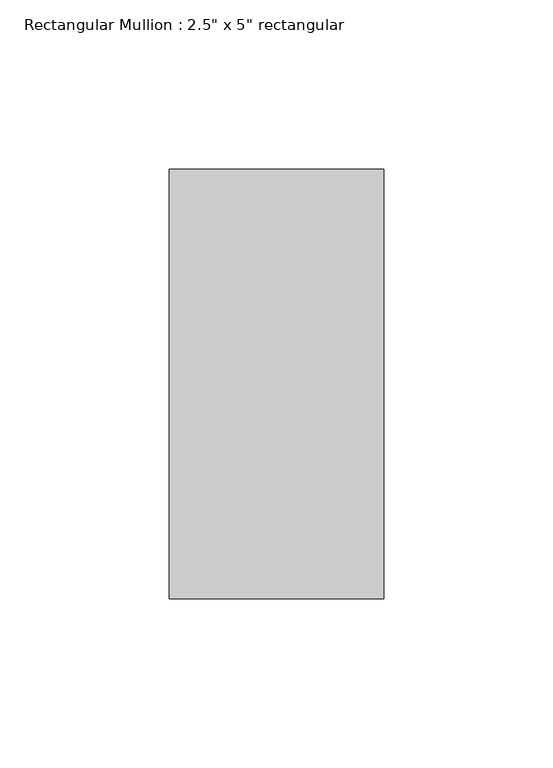
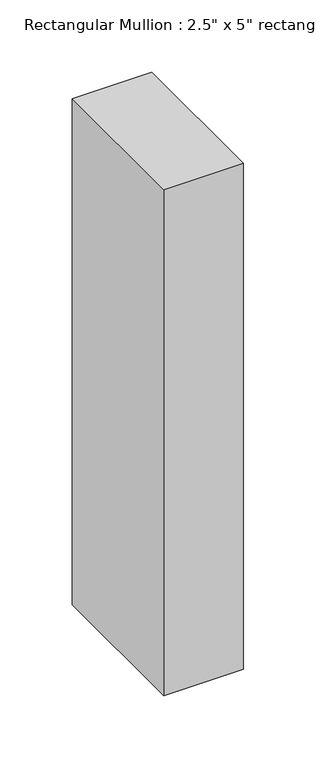
"""IFC4 building model written with IfcOpenShell, lengths in millimetres: member geometry."""

from ifc_helpers import new_model, si_unit, frame, origin, place, context, project, spatial, polyline, outline, extrude, source, transform, mapped, element, save


def member_cf238b44(model_context):
    return source(origin(), model_context, "Body", "SweptSolid", [
        extrude(outline(polyline([(31.75, 63.5), (31.75, -63.5), (-31.75, -63.5), (-31.75, 63.5), (31.75, 63.5)])), frame((0.0, 0.0, -427.5666667), z_axis=(0.0, 0.0, 1.0), x_axis=(1.0, 0.0, 0.0)), (0.0, 0.0, 1.0), 427.5666667),
    ])


if __name__ == "__main__":
    model = new_model("IFC4")
    model_context = context("Model", 3, world=origin())
    ifc_project = project(units=[si_unit("LENGTHUNIT", "METRE", prefix="MILLI")], contexts=[model_context])
    site = spatial("IfcSite", under=ifc_project)
    building = spatial("IfcBuilding", under=site)
    placement = place(None, origin())
    member_shape = member_cf238b44(model_context)
    element("IfcMember", 1, ObjectType="Rectangular Mullion : 2.5\" x 5\" rectangular", at=placement, inside=building, context=model_context, shape_type="MappedRepresentation", body=[
        mapped(member_shape, transform((0.0, 0.0, 0.0), x_axis=(1.0, 0.0, 0.0), y_axis=(0.0, 1.0, 0.0), z_axis=(0.0, 0.0, 1.0))),
    ])
    save(model, "model.ifc")

# Revit data of these elements
# Type "Rectangular Mullion : 2.5\" x 5\" rectangular"
#   built-in parameter 1007304 = 0.416667 (stored number, unit not read)
#   built-in parameter 1007301 = 0.104167 (stored number, unit not read)
#   built-in parameter 1007300 = 0.104167 (stored number, unit not read)
